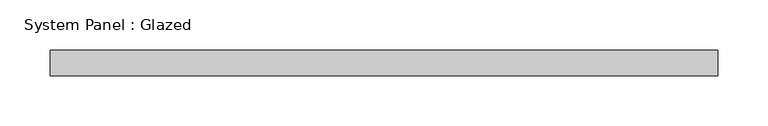
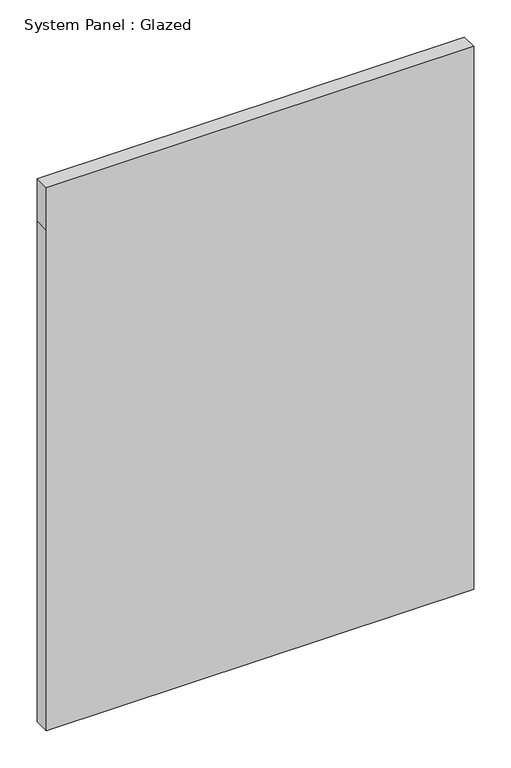
"""IFC4 building model written with IfcOpenShell, lengths in millimetres: plate geometry, System Panel : Glazed."""

from ifc_helpers import new_model, si_unit, frame, origin, place, context, project, spatial, polyline, outline, extrude, source, transform, mapped, element, save


def system_panel_glazed_cb6e72c2(model_context):
    return source(origin(), model_context, "Body", "SweptSolid", [
        extrude(outline(polyline([(0.0, -333.375), (0.0, 333.375), (826.1989237, 333.375), (896.0489237, 333.375), (896.0489237, -333.375), (826.1989237, -333.375), (0.0, -333.375)])), frame((0.0, 19.05, 0.0), z_axis=(0.0, 1.0, 0.0), x_axis=(0.0, 0.0, 1.0)), (0.0, 0.0, 1.0), 25.4),
    ])


if __name__ == "__main__":
    model = new_model("IFC4")
    model_context = context("Model", 3, world=origin())
    ifc_project = project(units=[si_unit("LENGTHUNIT", "METRE", prefix="MILLI")], contexts=[model_context])
    site = spatial("IfcSite", under=ifc_project)
    building = spatial("IfcBuilding", under=site)
    placement = place(None, origin())
    system_panel_glazed_shape = system_panel_glazed_cb6e72c2(model_context)
    element("IfcPlate", 1, ObjectType="System Panel : Glazed", at=placement, inside=building, context=model_context, shape_type="MappedRepresentation", body=[
        mapped(system_panel_glazed_shape, transform((0.0, 0.0, 0.0), x_axis=(1.0, 0.0, 0.0), y_axis=(0.0, 1.0, 0.0), z_axis=(0.0, 0.0, 1.0))),
    ])
    save(model, "model.ifc")

# Revit data of these elements
# Type "System Panel : Glazed"
#   Construction Type Id = "GSP4R"
#   Analytic Construction = "1/8 in Pilkington single glazing"
#   Visual Light Transmittance = 0.9
#   Solar Heat Gain Coefficient = 0.86
#   Heat Transfer Coefficient (U) = 1.18115 BTU/(h·ft²·°F)
#   Define Thermal Properties by = 1
# Element 1 (IfcPlate, "System Panel : Glazed")
#   Materials on its faces: "Glass"
# Materials
#   "Glass": class "Glass", colour RGB 0 128 192, transparency 0.75, Description = "Soda Lime Glass", Cost = 0
